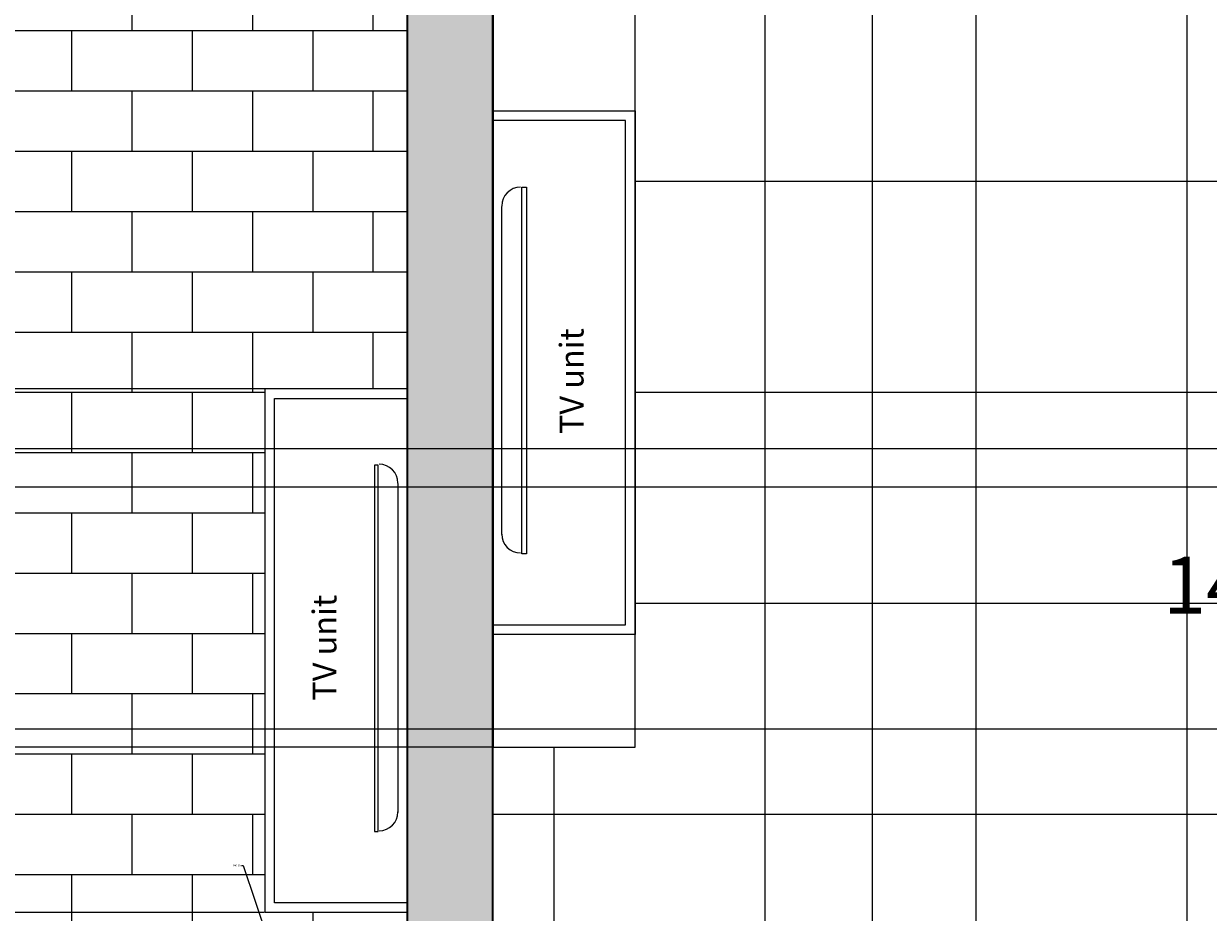
# Model space of a CAD drawing. Units: inches. Extents: x 6 to 575, y 34 to 566.
# Tile 5 of 21: x 157 to 282, y 293 to 387. Entities that reach past the tile are written whole.
import ezdxf

# ---------------------------------------------------------------- set-up
doc = ezdxf.new("R2010")
doc.units = ezdxf.units.IN
for name, color, linetype, lineweight in [('A-ANNO-DIMS', 2, 'Continuous', 18), ('A-ANNO-TEXT', 6, 'Continuous', 18), ('A-AREA-IDEN', 6, 'Continuous', 20), ('A-EQPM', 2, 'Continuous', 18), ('A-FLOR-CASE', 2, 'Continuous', 18), ('A-FLOR-PATT', 252, 'Continuous', 9), ('A-WALL-PATT', 251, 'Continuous', 9), ('WALLS', 7, 'Continuous', 35)]:
    doc.layers.add(name, color=color, linetype=linetype, lineweight=lineweight)
doc.styles.add('PDF Arial Narrow', font='txt')
doc.styles.add('PDF Century Gothic', font='txt')
doc.styles.get("Standard").update_dxf_attribs({"font": 'arial.ttf'})
doc.dimstyles.get("Standard").update_dxf_attribs({"dimtxt": 0.18, "dimasz": 0.18, "dimexe": 0.18, "dimexo": 0.0625, "dimgap": 0.09, "dimtad": 0, "dimtih": 1, "dimtoh": 1, "dimdec": 4, "dimzin": 0, "dimdsep": 46, "dimtxsty": 'Standard', "dimcen": 0.09, "dimadec": 0, "dimazin": 0, "dimtfac": 1, "dimtdec": 4, "dimtofl": 0, "dimtmove": 0, "dimatfit": 3, "dimfxl": 1, "dimtolj": 1, "dimtzin": 0, "dimarcsym": 0})

# ---------------------------------------------------------------- blocks, each defined once
blk = doc.blocks.new('*D30')
at = {"layer": 'A-ANNO-DIMS', "color": 0, "lineweight": -2, "transparency": 16777216}
for p, q in [((32.6, 539.8), (6.65, 539.8)), ((6.83, 539.62), (6.83, 299.97)), ((6.83, 59.95), (6.83, 299.61)), ((197.62, 59.77), (6.65, 59.77))]:
    blk.add_line(p, q, dxfattribs=at)
at = {"layer": 'A-ANNO-DIMS', "color": 0, "transparency": 16777216}
for points in [[(6.8, 539.62), (6.86, 539.62), (6.83, 539.8)], [(6.8, 59.95), (6.86, 59.95), (6.83, 59.77)]]:
    blk.add_solid(points, dxfattribs=at)
at = {"layer": 'Defpoints', "color": 0, "transparency": 16777216}
for p in [(32.66, 539.8), (6.83, 59.77), (197.69, 59.77)]:
    blk.add_point(p, dxfattribs=at)
at = {"layer": 'A-ANNO-DIMS', "color": 0, "transparency": 16777216, "insert": (6.83, 299.79), "char_height": 0.18, "attachment_point": 5}
blk.add_mtext('\\A1;480', dxfattribs=at)
blk = doc.blocks.new('*D54')
at = {"layer": 'A-ANNO-DIMS', "color": 0, "lineweight": -2, "transparency": 16777216}
for p, q in [((444.96, 337.94), (6.65, 337.94)), ((6.83, 337.76), (6.83, 299.11)), ((6.83, 260.1), (6.83, 298.75)), ((444.96, 259.92), (6.65, 259.92))]:
    blk.add_line(p, q, dxfattribs=at)
at = {"layer": 'A-ANNO-DIMS', "color": 0, "transparency": 16777216}
for points in [[(6.8, 337.76), (6.86, 337.76), (6.83, 337.94)], [(6.8, 260.1), (6.86, 260.1), (6.83, 259.92)]]:
    blk.add_solid(points, dxfattribs=at)
at = {"layer": 'Defpoints', "color": 0, "transparency": 16777216}
for p in [(6.83, 337.94), (445.02, 337.94), (445.02, 259.92)]:
    blk.add_point(p, dxfattribs=at)
at = {"layer": 'A-ANNO-DIMS', "color": 0, "transparency": 16777216, "insert": (6.83, 298.93), "char_height": 0.18, "attachment_point": 5}
blk.add_mtext('\\A1;78.02', dxfattribs=at)
blk = doc.blocks.new('*D59')
at = {"layer": 'A-ANNO-DIMS', "color": 0, "lineweight": -2, "transparency": 16777216}
for p, q in [((206.66, 224.86), (206.66, 565.81)), ((206.84, 565.63), (226.44, 565.63)), ((246.48, 565.63), (226.88, 565.63)), ((246.66, 224.86), (246.66, 565.81))]:
    blk.add_line(p, q, dxfattribs=at)
at = {"layer": 'A-ANNO-DIMS', "color": 0, "transparency": 16777216}
for points in [[(206.84, 565.66), (206.84, 565.6), (206.66, 565.63)], [(246.48, 565.66), (246.48, 565.6), (246.66, 565.63)]]:
    blk.add_solid(points, dxfattribs=at)
at = {"layer": 'Defpoints', "color": 0, "transparency": 16777216}
for p in [(246.66, 565.63), (206.66, 224.8), (246.66, 224.8)]:
    blk.add_point(p, dxfattribs=at)
at = {"layer": 'A-ANNO-DIMS', "color": 0, "transparency": 16777216, "insert": (226.66, 565.63), "char_height": 0.18, "attachment_point": 5}
blk.add_mtext('\\A1;40', dxfattribs=at)
blk = doc.blocks.new('*D104')
at = {"layer": 'A-ANNO-DIMS', "color": 0, "lineweight": -2, "transparency": 16777216}
for p, q in [((197.64, 348.32), (6.65, 348.32)), ((6.83, 348.14), (6.83, 320.93)), ((6.83, 293.34), (6.83, 320.56)), ((182.58, 293.16), (6.65, 293.16))]:
    blk.add_line(p, q, dxfattribs=at)
at = {"layer": 'A-ANNO-DIMS', "color": 0, "transparency": 16777216}
for points in [[(6.8, 348.14), (6.86, 348.14), (6.83, 348.32)], [(6.8, 293.34), (6.86, 293.34), (6.83, 293.16)]]:
    blk.add_solid(points, dxfattribs=at)
at = {"layer": 'Defpoints', "color": 0, "transparency": 16777216}
for p in [(6.83, 348.32), (197.7, 348.32), (182.64, 293.16)]:
    blk.add_point(p, dxfattribs=at)
at = {"layer": 'A-ANNO-DIMS', "color": 0, "transparency": 16777216, "insert": (6.83, 320.74), "char_height": 0.18, "attachment_point": 5}
blk.add_mtext('\\A1;55.16', dxfattribs=at)
blk = doc.blocks.new('*D132')
at = {"layer": 'A-ANNO-DIMS', "color": 0, "lineweight": -2, "transparency": 16777216}
for p, q in [((288.54, 390), (6.65, 390)), ((6.83, 389.82), (6.83, 366.19)), ((6.83, 342.19), (6.83, 365.82)), ((288.54, 342.01), (6.65, 342.01))]:
    blk.add_line(p, q, dxfattribs=at)
at = {"layer": 'A-ANNO-DIMS', "color": 0, "transparency": 16777216}
for points in [[(6.8, 389.82), (6.86, 389.82), (6.83, 390)], [(6.8, 342.19), (6.86, 342.19), (6.83, 342.01)]]:
    blk.add_solid(points, dxfattribs=at)
at = {"layer": 'Defpoints', "color": 0, "transparency": 16777216}
for p in [(6.83, 390), (288.6, 390), (288.6, 342.01)]:
    blk.add_point(p, dxfattribs=at)
at = {"layer": 'A-ANNO-DIMS', "color": 0, "transparency": 16777216, "insert": (6.83, 366), "char_height": 0.18, "attachment_point": 5}
blk.add_mtext('\\A1;47.98', dxfattribs=at)
blk = doc.blocks.new('*D133')
at = {"layer": 'A-ANNO-DIMS', "color": 0, "lineweight": -2, "transparency": 16777216}
for p, q in [((288.54, 342.01), (6.65, 342.01)), ((6.83, 341.83), (6.83, 327.42)), ((6.83, 312.63), (6.83, 327.05)), ((288.79, 312.45), (6.65, 312.45))]:
    blk.add_line(p, q, dxfattribs=at)
at = {"layer": 'A-ANNO-DIMS', "color": 0, "transparency": 16777216}
for points in [[(6.8, 341.83), (6.86, 341.83), (6.83, 342.01)], [(6.8, 312.63), (6.86, 312.63), (6.83, 312.45)]]:
    blk.add_solid(points, dxfattribs=at)
at = {"layer": 'Defpoints', "color": 0, "transparency": 16777216}
for p in [(288.6, 342.01), (6.83, 312.45), (288.86, 312.45)]:
    blk.add_point(p, dxfattribs=at)
at = {"layer": 'A-ANNO-DIMS', "color": 0, "transparency": 16777216, "insert": (6.83, 327.23), "char_height": 0.18, "attachment_point": 5}
blk.add_mtext('\\A1;29.56', dxfattribs=at)
blk = doc.blocks.new('*D136')
at = {"layer": 'A-ANNO-DIMS', "color": 0, "lineweight": -2, "transparency": 16777216}
for p, q in [((206.62, 389.45), (6.65, 389.45)), ((6.83, 389.27), (6.83, 350.19)), ((6.83, 310.75), (6.83, 349.83)), ((206.62, 310.57), (6.65, 310.57))]:
    blk.add_line(p, q, dxfattribs=at)
at = {"layer": 'A-ANNO-DIMS', "color": 0, "transparency": 16777216}
for points in [[(6.8, 389.27), (6.86, 389.27), (6.83, 389.45)], [(6.8, 310.75), (6.86, 310.75), (6.83, 310.57)]]:
    blk.add_solid(points, dxfattribs=at)
at = {"layer": 'Defpoints', "color": 0, "transparency": 16777216}
for p in [(6.83, 389.45), (206.68, 389.45), (206.68, 310.57)]:
    blk.add_point(p, dxfattribs=at)
at = {"layer": 'A-ANNO-DIMS', "color": 0, "transparency": 16777216, "insert": (6.83, 350.01), "char_height": 0.18, "attachment_point": 5}
blk.add_mtext('\\A1;78.88', dxfattribs=at)
blk = doc.blocks.new('*D137')
at = {"layer": 'A-ANNO-DIMS', "color": 0, "lineweight": -2, "transparency": 16777216}
for p, q in [((206.62, 310.57), (6.65, 310.57)), ((6.83, 310.39), (6.83, 267.87)), ((6.83, 224.98), (6.83, 267.5)), ((206.6, 224.8), (6.65, 224.8))]:
    blk.add_line(p, q, dxfattribs=at)
at = {"layer": 'A-ANNO-DIMS', "color": 0, "transparency": 16777216}
for points in [[(6.8, 310.39), (6.86, 310.39), (6.83, 310.57)], [(6.8, 224.98), (6.86, 224.98), (6.83, 224.8)]]:
    blk.add_solid(points, dxfattribs=at)
at = {"layer": 'Defpoints', "color": 0, "transparency": 16777216}
for p in [(6.83, 310.57), (206.68, 310.57), (206.66, 224.8)]:
    blk.add_point(p, dxfattribs=at)
at = {"layer": 'A-ANNO-DIMS', "color": 0, "transparency": 16777216, "insert": (6.83, 267.69), "char_height": 0.18, "attachment_point": 5}
blk.add_mtext('\\A1;85.77', dxfattribs=at)
blk = doc.blocks.new('*D228')
at = {"layer": 'A-ANNO-DIMS', "color": 0, "lineweight": -2, "transparency": 16777216}
for p, q in [((180.18, 298.09), (180.36, 298.09)), ((180.36, 298.09), (188.66, 273.48)), ((202.66, 231.92), (202.66, 232.1)), ((202.57, 232.01), (202.75, 232.01))]:
    blk.add_line(p, q, dxfattribs=at)
at = {"layer": 'A-ANNO-DIMS', "color": 0, "transparency": 16777216}
blk.add_solid([(188.69, 273.49), (188.64, 273.47), (188.72, 273.31)], dxfattribs=at)
at = {"layer": 'Defpoints', "color": 0, "transparency": 16777216}
for p in [(188.72, 273.31), (202.66, 232.01)]:
    blk.add_point(p, dxfattribs=at)
at = {"layer": 'A-ANNO-DIMS', "color": 0, "transparency": 16777216, "insert": (179.7, 298.09), "char_height": 0.18, "attachment_point": 5}
blk.add_mtext('\\A1;R43.59', dxfattribs=at)

msp = doc.modelspace()

# ---------------------------------------------------------------- hatches: boundary and pattern name
at = {"layer": 'A-FLOR-PATT'}
h = msp.add_hatch(dxfattribs=at)
h.set_pattern_fill('BRICK', color=256)
h.set_pattern_definition([(0, (-98.035, 170.1465), (0, 6.35), []), (90, (-98.035, 170.147), (-12.7, 8e-16), [6.35, -6.35]), (90, (-91.685, 170.147), (-12.7, 8e-16), [-6.35, 6.35])])
h.paths.add_polyline_path([(180.8711, 269.7588), (182.4439, 270.6668), (182.4628, 270.6341, -0.11619827), (201.8275, 275.5902), (201.8275, 276.801), (197.6586, 276.801), (197.6586, 293.1641), (182.6401, 293.1641), (182.6401, 348.324), (197.6586, 348.324), (197.6586, 407.7709), (112.8513, 407.7709), (112.8513, 431.801), (111.6586, 431.801), (111.6586, 440.801), (117.6586, 440.801), (117.6586, 446.801), (117.6586, 448.2751), (117.6586, 473.3269), (117.6586, 474.801), (117.6586, 515.5941), (100.2533, 515.5941, -1), (83.0548, 515.5941), (65.6494, 515.5941), (65.6494, 440.801), (82.8918, 440.801), (82.8918, 431.801), (82.8918, 407.7709), (41.6586, 407.7709), (41.6586, 379.0637), (62.6459, 379.0637), (62.6459, 358.0764), (122.565, 358.0764), (122.565, 286.0643), (62.6459, 286.0643), (62.6459, 265.077), (41.6586, 265.077), (41.6586, 224.801), (41.6586, 212.801), (71.6586, 212.801), (167.6586, 212.801), (197.6586, 212.801), (197.6586, 230.801), (201.8157, 230.801), (201.8157, 233.4817)])
h.paths.add_polyline_path([(133.3414, 245.1275), (133.3317, 245.1352), (133.3317, 245.104)], flags=16)
h.paths.add_polyline_path([(133.3317, 222.1662), (85.3496, 222.1662), (85.3496, 243.7443, -0.50090726), (87.1831, 246.1963), (107.4292, 246.1963), (111.2522, 246.1963), (131.4202, 246.1963, -0.41421356), (133.3317, 244.2848)], flags=16)
h.paths.add_polyline_path([(72.7105, 244.4018), (72.7105, 220.3718), (48.6804, 220.3718), (48.6804, 244.4018)], flags=16)
h.paths.add_polyline_path([(71.7466, 237.8955, -1), (59.8096, 237.8955, -1)], flags=0)
h = msp.add_hatch(dxfattribs=at)
h.set_pattern_fill('NET', color=256, scale=7)
h.set_pattern_definition([(0, (-98.035, 170.147), (0, 22.225), []), (90, (-98.035, 170.147), (-22.225, 1e-15), [])])
h.paths.add_polyline_path([(368.183, 395.6385, -0.88370529), (374.2533, 394.8861), (374.6586, 448.801), (354.6586, 448.801), (354.6586, 448.7938), (353.1847, 448.7938), (326.6586, 448.801), (322.6586, 448.801), (248.6332, 448.8024), (206.6586, 448.8024), (206.6586, 389.449), (221.6622, 389.449), (221.6622, 310.5712), (206.6586, 310.5712), (206.6586, 276.801), (206.6704, 276.801), (206.6704, 274.3795), (206.6586, 224.801), (246.6586, 224.801), (264.6586, 224.801), (265.6986, 224.801), (265.6986, 249.081), (267.5186, 249.081), (267.5186, 249.0145, -0.38515288), (290.6494, 224.801), (290.6679, 224.801, -0.38515288), (313.7986, 249.0145), (313.7986, 249.081), (315.6186, 249.081), (315.6186, 224.801), (316.6586, 224.801), (334.6586, 224.801), (374.6586, 224.801), (374.6586, 278.801), (374.1753, 318.8919, -0.45530286), (370.7577, 315.9168), (370.6643, 313.8205, -0.41421356), (368.7528, 311.909), (368.8072, 311.8975), (368.7528, 311.909, 0.41421356), (370.6643, 313.8205), (370.7632, 315.9161, -0.34634601), (368.183, 318.5897)])
h.paths.add_polyline_path([(288.603, 342.0131), (288.603, 389.9952), (318.6406, 389.9952), (318.6406, 342.0131)], flags=16)
h.paths.add_polyline_path([(289.6173, 343.0274), (289.6173, 389.059), (317.6263, 389.059), (317.6263, 343.0274)], flags=0)
h.paths.add_polyline_path([(295.4867, 311.7535, 0.06538163), (295.1241, 312.0945), (295.0006, 312.1316)], flags=16)
h.paths.add_polyline_path([(328.4931, 284.9911, 0.41421356), (330.4045, 286.9026), (330.4215, 286.8532), (330.4045, 286.9026, -0.41421356), (328.4931, 284.9911), (328.549, 284.9808)], flags=16)
h.paths.add_polyline_path([(344.7771, 305.2659), (368.8072, 305.2659), (368.8072, 281.2358), (344.7771, 281.2358)], flags=16)
h.paths.add_polyline_path([(368.183, 288.1406, -1), (356.246, 288.1406, -1)], flags=0)
h.paths.add_polyline_path([(347.9759, 404.6629), (347.9759, 428.6929), (372.006, 428.6929), (372.006, 404.6629)], flags=16)
h.paths.add_polyline_path([(359.4448, 421.7882, -1), (371.3818, 421.7882, -1)], flags=0)
at = {"layer": 'A-WALL-PATT'}
h = msp.add_hatch(color=256, dxfattribs=at)
h.dxf.hatch_style = 1
h.paths.add_polyline_path([(160.6586, 539.801), (32.6586, 539.801), (32.6586, 272.801), (41.6586, 272.801), (41.6586, 286.0643), (41.6586, 358.0764), (41.6586, 379.0637), (41.6586, 407.7709), (41.6194, 407.7709), (41.6194, 431.801), (82.8918, 431.801), (82.8918, 440.801), (65.6494, 440.801), (65.6494, 440.7732), (41.6194, 440.7732), (41.6194, 515.5941), (41.6586, 530.801), (117.6586, 530.801), (117.6586, 474.801), (120.6068, 474.801), (121.6586, 474.801), (121.6586, 530.801), (137.4275, 530.801), (137.4275, 530.8356), (141.2505, 530.8356), (160.6586, 530.801)])
h.paths.add_polyline_path([(71.6586, 212.801), (41.6586, 212.801), (41.6586, 224.801), (32.6586, 224.801), (32.6586, 203.801), (71.6586, 203.801)])
h.paths.add_polyline_path([(206.6586, 215.801), (246.6586, 215.801), (246.6586, 224.801), (206.6586, 224.801), (206.6586, 230.801), (201.8157, 230.801), (197.6586, 230.801), (197.6586, 212.801), (167.6586, 212.801), (167.6586, 203.801), (206.6586, 203.801)])
h.paths.add_polyline_path([(383.6586, 224.801), (334.6586, 224.801), (334.6586, 215.801), (374.6586, 215.801), (374.6586, 203.801), (384.0753, 203.801), (407.6586, 203.801), (407.6586, 212.801), (383.6586, 212.801)])
h.paths.add_polyline_path([(548.6586, 270.801), (539.6586, 270.801), (539.6586, 212.801), (515.6586, 212.801), (515.6586, 203.801), (548.6586, 203.801)])
h.paths.add_polyline_path([(548.6586, 412.801), (545.7108, 412.801), (539.6586, 412.801), (539.6586, 382.801), (433.708, 382.801), (433.708, 378.801), (539.6586, 378.801), (539.6586, 366.801), (548.6586, 366.801)])
h.paths.add_polyline_path([(548.6586, 539.801), (455.9436, 539.801), (455.9436, 530.801), (539.6586, 530.801), (539.6586, 440.801), (548.6586, 440.801)])
h.paths.add_polyline_path([(407.9436, 539.801), (362.6586, 539.801), (362.6586, 530.801), (374.6586, 530.801), (374.6586, 452.801), (354.6586, 452.801), (354.6586, 448.801), (374.6586, 448.801), (374.6586, 278.801), (383.6586, 278.801), (383.6586, 530.801), (407.9436, 530.801)])
h.paths.add_polyline_path([(338.6586, 539.801), (320.6586, 539.801), (320.6586, 530.801), (322.6586, 530.801), (322.6586, 448.801), (326.6586, 448.801), (326.6586, 530.801), (338.6586, 530.801)])
h.paths.add_polyline_path([(272.6586, 539.801), (184.6586, 539.801), (184.6586, 530.801), (197.6586, 530.801), (197.6586, 440.801), (176.6714, 440.801), (121.6586, 440.801), (121.6586, 446.801), (117.6586, 446.801), (117.6586, 440.801), (111.6586, 440.801), (111.6586, 431.801), (197.6586, 431.801), (197.6586, 407.7709), (197.6586, 276.801), (206.6586, 276.801), (206.6586, 530.801), (272.6586, 530.801)])

# ---------------------------------------------------------------- linework, layer by layer
at = {"layer": 'A-EQPM'}
for points in [[(210.1933, 330.9343), (209.7252, 330.9343), (209.7252, 369.554), (210.1933, 369.554)], [(194.187, 301.6682), (194.5771, 301.6682), (194.5771, 340.288), (194.187, 340.288)]]:
    msp.add_lwpolyline(points, close=True, dxfattribs=at)
for points in [[(207.6186, 332.9628), (207.6186, 367.5255)], [(196.6836, 303.6968), (196.6836, 338.3375)]]:
    msp.add_lwpolyline(points, dxfattribs=at)
for centre, start, end in [((209.5863, 367.5782), 90.000003, 179.999997), ((194.6717, 338.3888), 0, 89.999997), ((209.5863, 333.0141), 180.000003, 269.999997), ((194.6717, 303.7467), 270.000003, 359.999997)]:
    msp.add_arc(centre, 1.9895, start, end, dxfattribs=at)
at = {"layer": 'A-FLOR-CASE'}
for points in [[(206.6824, 389.449), (206.6824, 310.5712), (221.6622, 310.5712), (221.6622, 389.449)], [(206.6824, 310.5712), (221.6622, 310.5712), (221.6622, 322.4302), (206.6824, 322.4302)]]:
    msp.add_lwpolyline(points, close=True, dxfattribs=at)
for points in [[(206.6824, 377.5901), (221.6622, 377.5901), (221.6622, 322.4302), (206.6824, 322.4302)], [(206.6824, 323.4444), (220.6479, 323.4444), (220.6479, 376.5758), (206.6824, 376.5758)], [(197.6979, 348.324), (182.6401, 348.324), (182.6401, 293.1641), (197.6979, 293.1641)], [(197.6979, 294.1784), (183.6544, 294.1784), (183.6544, 347.3097), (197.6979, 347.3097)]]:
    msp.add_lwpolyline(points, dxfattribs=at)
at = {"layer": 'WALLS'}
for p, q in [((206.6586, 276.801), (206.6586, 530.801)), ((197.6586, 276.801), (197.6586, 431.801))]:
    msp.add_line(p, q, dxfattribs=at)

# ---------------------------------------------------------------- texts
at = {"layer": 'A-ANNO-TEXT', "char_height": 2.50021, "attachment_point": 4, "rotation": 90, "style": 'PDF Century Gothic'}
for insert in [(215.2887, 343.5574), (189.2607, 315.4692)]:
    msp.add_mtext('TV unit', dxfattribs=dict(at, insert=insert))
at = {"layer": 'A-AREA-IDEN', "insert": (277.2546, 326.8505), "char_height": 6.000503, "attachment_point": 4, "style": 'PDF Arial Narrow'}
msp.add_mtext('14\'-0" X 18\'-8"', dxfattribs=at)

# ---------------------------------------------------------------- dimensions: what is measured, and where the dimension line sits
at = {"layer": 'A-ANNO-DIMS'}
dim = msp.add_linear_dim(base=(246.6586, 565.631), p1=(206.6586, 224.801), p2=(246.6586, 224.801), dimstyle='Standard', override={"dimdec": 0, "dimlfac": 1, "dimrnd": 0, "dimzin": 0, "dimdsep": 46, "dimlunit": 2}, dxfattribs=at)
dim.commit()
dim.dimension.update_dxf_attribs({"geometry": '*D59', "text_midpoint": (226.6586, 565.631)})
for base, p1, p2, override, picture, middle in [((6.8286, 59.7747), (32.6586, 539.801), (197.6872, 59.7747), {"dimdec": 0, "dimlfac": 1, "dimrnd": 0, "dimzin": 0, "dimdsep": 46, "dimlunit": 2}, '*D30', (6.8286, 299.7878)), ((6.8286, 389.9952), (288.603, 342.0131), (288.603, 389.9952), {"dimdec": 2, "dimlfac": 1, "dimrnd": 0, "dimzin": 0, "dimdsep": 46, "dimlunit": 2}, '*D132', (6.8286, 366.0042)), ((6.8286, 389.449), (206.6824, 310.5712), (206.6824, 389.449), {"dimdec": 2, "dimlfac": 1, "dimrnd": 0, "dimzin": 0, "dimdsep": 46, "dimlunit": 2}, '*D136', (6.8286, 350.0101)), ((6.8286, 348.324), (182.6401, 293.1641), (197.6979, 348.324), {"dimdec": 2, "dimlfac": 1, "dimrnd": 0, "dimzin": 0, "dimdsep": 46, "dimlunit": 2}, '*D104', (6.8286, 320.744)), ((6.8286, 312.455), (288.603, 342.0131), (288.8575, 312.455), {"dimdec": 2, "dimlfac": 1, "dimrnd": 0, "dimzin": 0, "dimdsep": 46, "dimlunit": 2}, '*D133', (6.8286, 327.234)), ((6.8286, 337.9397), (445.0208, 259.9201), (445.0208, 337.9397), {"dimdec": 2, "dimlfac": 1, "dimrnd": 0, "dimzin": 0, "dimdsep": 46, "dimlunit": 2}, '*D54', (6.8286, 298.9299)), ((6.8286, 310.5712), (206.6586, 224.801), (206.6824, 310.5712), {"dimdec": 2, "dimlfac": 1, "dimrnd": 0, "dimzin": 0, "dimdsep": 46, "dimlunit": 2}, '*D137', (6.8286, 267.6861))]:
    dim = msp.add_linear_dim(base=base, p1=p1, p2=p2, angle=90, dimstyle='Standard', override=override, dxfattribs=at)
    dim.commit()
    dim.dimension.update_dxf_attribs({"geometry": picture, "text_midpoint": middle})
dim = msp.add_radius_dim(center=(202.6644, 232.0117), mpoint=(188.7219, 273.3082), dimstyle='Standard', override={"dimdec": 2, "dimlfac": 1, "dimrnd": 0, "dimzin": 0, "dimdsep": 46, "dimlunit": 2}, dxfattribs=at)
dim.commit()
dim.dimension.update_dxf_attribs({"geometry": '*D228', "text_midpoint": (179.6965, 298.086), "dimtype": 164})

doc.saveas('drawing.dxf')
